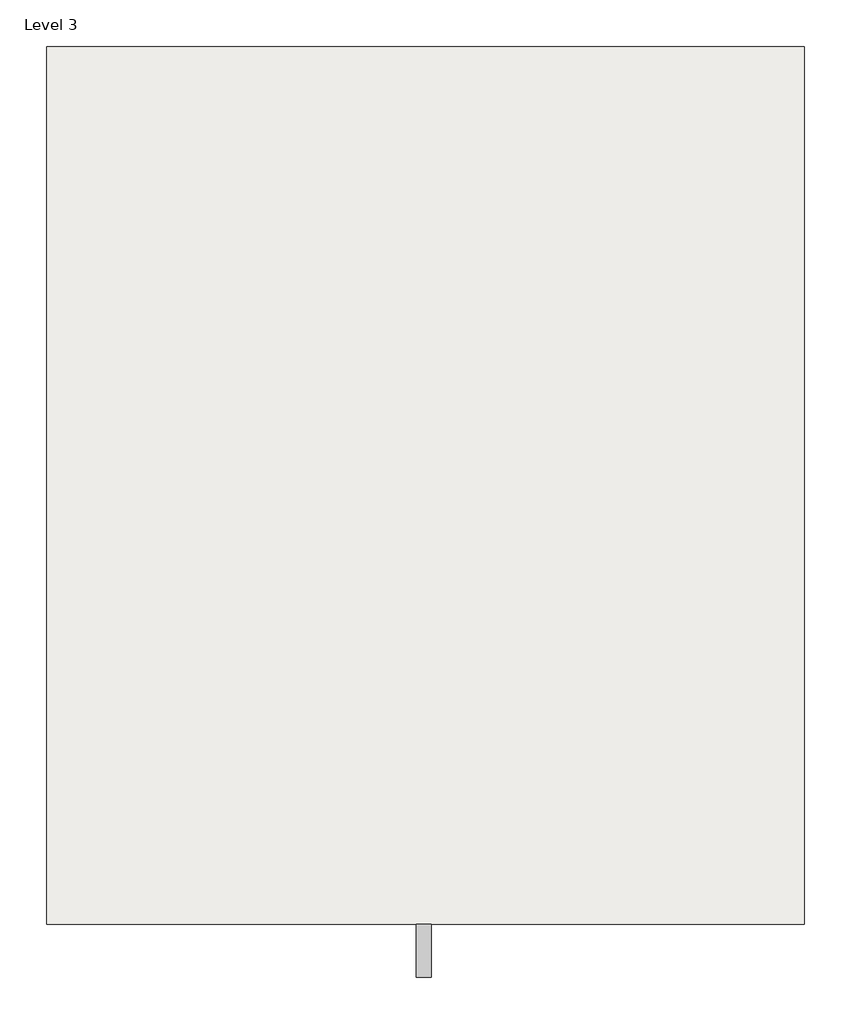
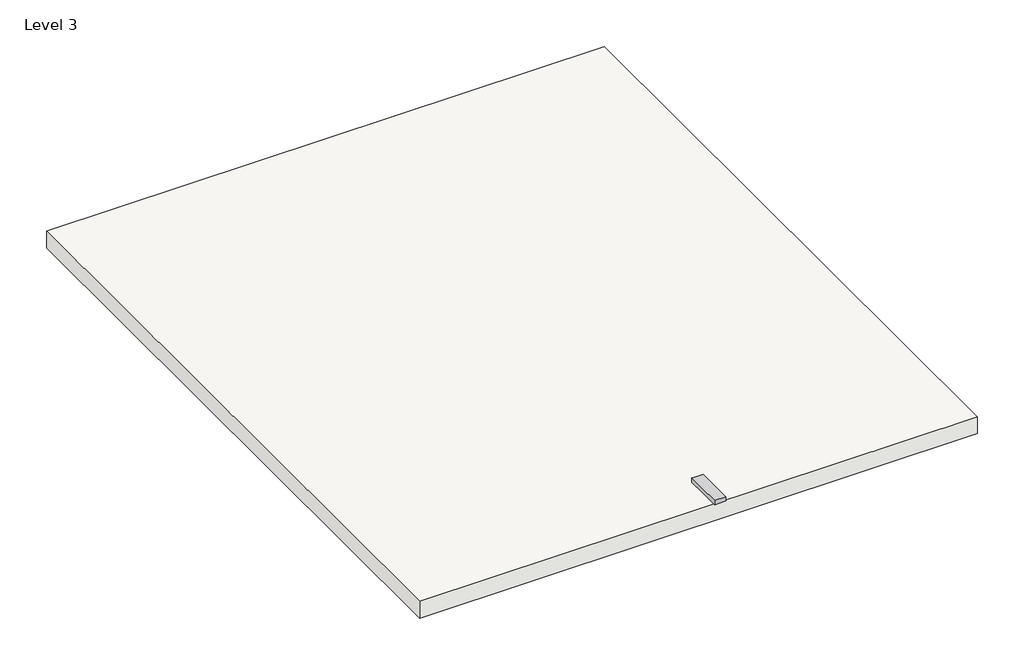
# One storey: 1 proxy, 1 roof.
"""IFC4 building model written with IfcOpenShell, lengths in millimetres."""

from ifc_helpers import new_model, si_unit, frame, origin, place, context, project, spatial, polyline, outline, extrude, transform, mapped, element, save
from components import generic_models_4_generic_models_4_66c3474a

model = new_model("IFC4")

# Units and contexts
model_context = context("Model", 3, world=origin())
ifc_project = project(units=[si_unit("LENGTHUNIT", "METRE", prefix="MILLI")], contexts=[model_context])

# Site, building, storey
site = spatial("IfcSite", under=ifc_project)
building = spatial("IfcBuilding", under=site)
storey = spatial("IfcBuildingStorey", under=building, Name="Level 3", Elevation=6096.0)

# Proxy
placement = place(None, origin())
generic_models_4_generic_models_4_shape = generic_models_4_generic_models_4_66c3474a(model_context)
element("IfcBuildingElementProxy", 1, Name="Generic Models 4 : Generic Models 4", ObjectType="Generic Models 4 : Generic Models 4", at=placement, inside=storey, context=model_context, shape_type="MappedRepresentation", body=[
    mapped(generic_models_4_generic_models_4_shape, transform((0.0, 0.0, 0.0), x_axis=(1.0, 0.0, 0.0), y_axis=(0.0, 1.0, 0.0), z_axis=(0.0, 0.0, 1.0))),
])

# Roof
element("IfcRoof", 2, ObjectType="Generic - 12\"", at=placement, inside=storey, context=model_context, shape_type="SweptSolid", body=[
    extrude(outline(polyline([(-17585.2518575, -4029.5378384), (-7984.0518575, -4029.5378384), (-7984.0518575, -15154.7378384), (-17585.2518575, -15154.7378384), (-17585.2518575, -4029.5378384)])), frame((0.0, 0.0, 6096.0), z_axis=(0.0, 0.0, 1.0), x_axis=(1.0, 0.0, 0.0)), (0.0, 0.0, 1.0), 304.8),
])

save(model, "model.ifc")

# Revit data of these elements
# Type "Generic - 12\""
#   Assembly Code = "B1020"
#   Layers, outside or top first: 1' - 0" no material (function 1)
# Element 1 (IfcBuildingElementProxy, "Generic Models 4 : Generic Models 4")
#   Phase Created = New Construction
# Element 2 (IfcRoof, "Generic - 12\"")
#   built-in parameter 1001705 = 21 (stored number, unit not read)
#   built-in parameter 1001710 = 33615
#   Phase Created = New Construction
#   Materials on its faces: "Default Roof"
# Materials
#   "Default Roof": colour RGB 88 101 114, transparency 0, Cost = 0
